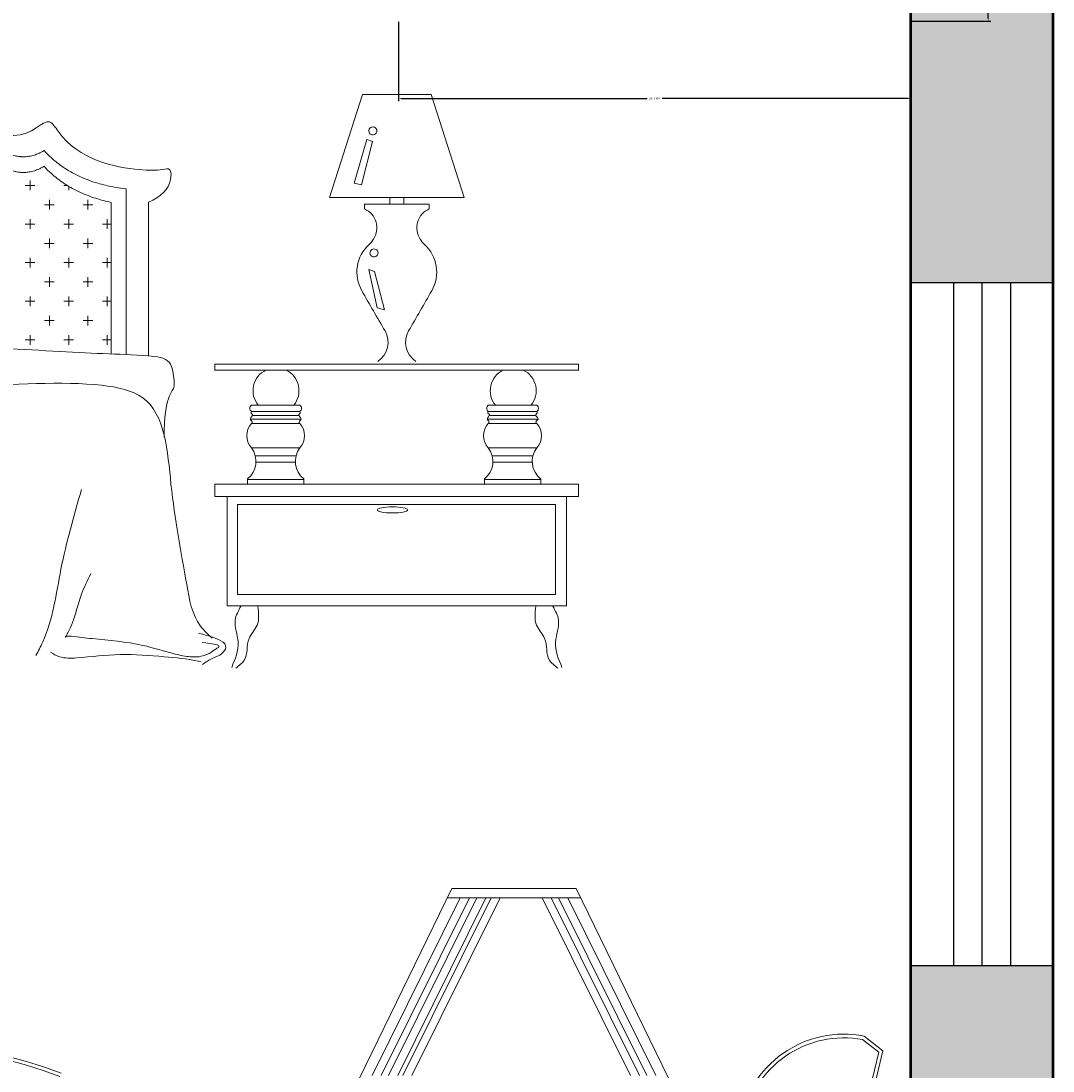
# Model space of a CAD drawing. Units: inches. Extents: x 1771 to 3025, y 319 to 889.
# Tile 34 of 35: x 2952 to 3025, y 714 to 788. Entities that reach past the tile are written whole.
import ezdxf

# ---------------------------------------------------------------- set-up
doc = ezdxf.new("R2010")
doc.units = ezdxf.units.IN
doc.header["$MEASUREMENT"] = 0
doc.set_wipeout_variables(frame=1)
for name, color, linetype, lineweight in [('A-ANNO-DIMS', 2, 'Continuous', 18), ('A-FURN', 8, 'Continuous', 18), ('A-GLAZ', 40, 'Continuous', 25), ('A-WALL', 7, 'Continuous', 50), ('A-WALL-PATT', 254, 'Continuous', 13)]:
    doc.layers.add(name, color=color, linetype=linetype, lineweight=lineweight)
doc.styles.get("Standard").update_dxf_attribs({"font": 'arial.ttf'})
doc.dimstyles.get("Standard").update_dxf_attribs({"dimtxt": 0.18, "dimasz": 0.18, "dimexe": 0.18, "dimexo": 0.0625, "dimgap": 0.09, "dimtad": 0, "dimtih": 1, "dimtoh": 1, "dimdec": 4, "dimzin": 0, "dimdsep": 46, "dimtxsty": 'Standard', "dimcen": 0.09, "dimadec": 0, "dimazin": 0, "dimtfac": 1, "dimtdec": 4, "dimtofl": 0, "dimtmove": 0, "dimatfit": 3, "dimfxl": 1, "dimtolj": 1, "dimtzin": 0, "dimarcsym": 0})

# ---------------------------------------------------------------- blocks, each defined once
blk = doc.blocks.new('A$C3F6F0378')
for p, q in [((2294.6, 774.2), (2348.7, 943.6)), ((2462.2, 943.6), (2348.7, 943.6)), ((2516.4, 774.2), (2462.2, 943.6)), ((2335.1, 797.8), (2356.3, 869.3)), ((2365.5, 866.2), (2347.3, 794.8)), ((2356.3, 869.3), (2365.5, 866.2)), ((1801.9, 785.9), (1801.9, 801.8)), ((2347.3, 794.8), (2335.1, 797.8)), ((1794, 793.9), (1809.9, 793.9)), ((1857.5, 793.9), (1863, 793.9)), ((1865.4, 785.9), (1865.4, 792.4)), ((1825.7, 762.1), (1841.6, 762.1)), ((1833.7, 754.2), (1833.7, 770)), ((1889.2, 762.1), (1905.1, 762.1)), ((1897.2, 754.2), (1897.2, 770)), ((2516.4, 774.2), (2294.6, 774.2)), ((2352.3, 763), (2352.3, 755.2)), ((2352.3, 763), (2352.3, 755.2)), ((2458.6, 763), (2352.3, 763)), ((2393.8, 774.2), (2393.8, 763)), ((2417.1, 763), (2393.8, 763)), ((2417.1, 774.2), (2417.1, 763)), ((2458.6, 763), (2458.6, 755.2)), ((2458.6, 763), (2458.6, 755.2)), ((1794, 730.4), (1809.9, 730.4)), ((1801.9, 722.4), (1801.9, 738.3)), ((1857.5, 730.4), (1873.4, 730.4)), ((1865.4, 722.4), (1865.4, 738.3)), ((1921, 730.4), (1935.3, 730.4)), ((1928.9, 722.4), (1928.9, 738.3)), ((1825.7, 698.6), (1841.6, 698.6)), ((1833.7, 690.7), (1833.7, 706.5)), ((1889.2, 698.6), (1905.1, 698.6)), ((1897.2, 690.7), (1897.2, 706.5)), ((1801.9, 658.9), (1801.9, 674.8)), ((1865.4, 658.9), (1865.4, 674.8)), ((1928.9, 658.9), (1928.9, 674.8)), ((1794, 666.9), (1809.9, 666.9)), ((1857.5, 666.9), (1873.4, 666.9)), ((1921, 666.9), (1935.3, 666.9)), ((1833.7, 627.2), (1833.7, 643)), ((1897.2, 627.2), (1897.2, 643)), ((2359.5, 655.6), (2368.6, 652.5)), ((2373.2, 592.3), (2359.5, 655.6)), ((2368.6, 652.5), (2385.4, 589.2)), ((1825.7, 635.1), (1841.6, 635.1)), ((1889.2, 635.1), (1905.1, 635.1)), ((1801.9, 595.4), (1801.9, 611.3)), ((1865.4, 595.4), (1865.4, 611.3)), ((1928.9, 595.4), (1928.9, 611.3)), ((1794, 603.4), (1809.9, 603.4)), ((1857.5, 603.4), (1873.4, 603.4)), ((1921, 603.4), (1935.3, 603.4)), ((2385.4, 589.2), (2373.2, 592.3)), ((1825.7, 571.6), (1841.6, 571.6)), ((1833.7, 563.7), (1833.7, 579.5)), ((1889.2, 571.6), (1905.1, 571.6)), ((1897.2, 563.7), (1897.2, 579.5)), ((1794, 539.9), (1809.9, 539.9)), ((1801.9, 531.9), (1801.9, 547.8)), ((1857.5, 539.9), (1873.4, 539.9)), ((1865.4, 531.9), (1865.4, 547.8)), ((1921, 539.9), (1935.3, 539.9)), ((1928.9, 531.9), (1928.9, 547.8)), ((2704.5, 500), (2106.1, 500)), ((2106.1, 499.7), (2106.1, 489.7)), ((2704.5, 490), (2106.1, 490)), ((2704.5, 499.7), (2704.5, 489.7)), ((2246.1, 432.2), (2166.1, 432.2)), ((2246.1, 432.2), (2166.1, 432.2)), ((2635.9, 432.2), (2555.9, 432.2)), ((2635.9, 432.2), (2555.9, 432.2)), ((2246.1, 422.2), (2166.1, 422.2)), ((2244.2, 415.4), (2167.9, 415.4)), ((2635.9, 422.2), (2555.9, 422.2)), ((2634.1, 415.4), (2557.7, 415.4)), ((2248, 409.3), (2164.1, 409.3)), ((2246.1, 402.2), (2166.1, 402.2)), ((2637.9, 409.3), (2554, 409.3)), ((2635.9, 402.2), (2555.9, 402.2)), ((2246.1, 362.2), (2166.1, 362.2)), ((2239.7, 349.2), (2172.4, 349.2)), ((2635.9, 362.2), (2555.9, 362.2)), ((2629.6, 349.2), (2562.2, 349.2)), ((2238.5, 338.7), (2173.6, 338.7)), ((2628.4, 338.7), (2563.5, 338.7)), ((2159.8, 311), (2159.8, 302.2)), ((2252.3, 311), (2252.3, 302.2)), ((2549.7, 311), (2549.7, 302.2)), ((2642.2, 311), (2642.2, 302.2)), ((2106.1, 302.2), (2106.1, 282.2)), ((2704.5, 302.2), (2106.1, 302.2)), ((2252.3, 310.3), (2159.8, 310.3)), ((2186.1, 302.2), (2226.1, 302.2)), ((2186.1, 302.2), (2236.1, 302.2)), ((2642.2, 310.3), (2549.7, 310.3)), ((2575.9, 302.2), (2615.9, 302.2)), ((2575.9, 302.2), (2625.9, 302.2)), ((2704.5, 282.2), (2704.5, 302.2)), ((2704.5, 282.2), (2106.1, 282.2)), ((2126.1, 282.2), (2126.1, 102.2)), ((2684.5, 102.2), (2684.5, 282.2)), ((2143.3, 268.9), (2666.3, 268.9)), ((2143.3, 120.8), (2143.3, 268.9)), ((2666.3, 268.9), (2666.3, 120.8)), ((2666.3, 120.8), (2143.3, 120.8)), ((2126.1, 102.2), (2684.5, 102.2))]:
    blk.add_line(p, q)
at = {"ltscale": 20}
for p, q in [((1959.8, 788.3), (1959.8, 515.7)), ((1935.3, 766), (1935.3, 516.7)), ((1996.6, 766.2), (1996.6, 513.5))]:
    blk.add_line(p, q, dxfattribs=at)
for centre, radius, start, end in [((2365.7, 883.6), 6.48, 168.6084, 233.2112), ((2365.7, 883.6), 6.49, 104.0344, 168.6084), ((2366.1, 883.6), 6.51, 78.6968, 107.1924), ((2365.7, 883.9), 6.81, 278.2688, 342.9026), ((2366.1, 883.7), 6.5, 50.1648, 78.6968), ((2366.2, 883.8), 6.35, 342.9026, 50.1648), ((2365.7, 883.5), 6.42, 233.2112, 255.9722), ((2365.7, 883.8), 6.69, 255.9722, 278.2688), ((2338.7, 724.1), 33.9, 326.6744, 66.3416), ((2472.2, 724.1), 33.9, 113.6584, 213.3256), ((2401.2, 651.2), 61.5, 132.0366, 209.8723), ((2337, 722.3), 34.4, 312.0366, 330.6067), ((2473.8, 722.3), 34.4, 209.3933, 227.9634), ((2409.6, 651.2), 61.5, 330.1277, 47.9634), ((2367.7, 682.8), 6.48, 168.6084, 233.2112), ((2367.7, 682.8), 6.49, 104.0344, 168.6084), ((2367.7, 682.8), 6.42, 233.2112, 255.9722), ((2367.8, 683), 6.69, 255.9722, 278.2688), ((2368.1, 682.9), 6.51, 78.6968, 107.1924), ((2367.8, 683.1), 6.81, 278.2688, 342.9026), ((2368.1, 682.9), 6.5, 50.1648, 78.6968), ((2368.2, 683), 6.35, 342.9026, 50.1648), ((11218.8, 5715.8), 10230.1, 209.87228, 210.29853), ((-6408, 5715.8), 10230.1, 329.70147, 330.12772), ((2353.9, 535.9), 37.3, 302.5427, 30.2985), ((2457, 535.9), 37.3, 149.7015, 237.4573), ((2206.6, 456.1), 37.8, 115.9414, 219.2084), ((2206.6, 456.1), 37.8, 320.7916, 64.0586), ((2597, 456.1), 37.8, 115.9414, 219.2084), ((2597, 456.1), 37.8, 320.7916, 64.0586), ((2169.8, 427.2), 6.24, 126.78, 233.22), ((2242.3, 427.2), 6.24, 306.78, 53.22), ((2559.7, 427.2), 6.24, 126.78, 233.22), ((2632.2, 427.2), 6.24, 306.78, 53.22), ((2188.1, 382.2), 29.7, 137.7452, 222.2548), ((2224, 382.2), 29.7, 317.7452, 42.2548), ((2577.9, 382.2), 29.7, 137.7452, 222.2548), ((2613.9, 382.2), 29.7, 317.7452, 42.2548), ((2136.7, 339.8), 37, 308.7547, 37.2668), ((2275.4, 339.8), 37, 142.7332, 231.2453), ((2526.5, 339.8), 37, 308.7547, 37.2668), ((2665.3, 339.8), 37, 142.7332, 231.2453)]:
    blk.add_arc(centre, radius, start, end)
blk.add_ellipse((2398.3, 260.1), major_axis=(25, 0), ratio=0.2)
for points, knots in [([(1996.6, 766.2), (2017.1, 775.8), (2035.1, 791.6), (2033.8, 824.3), (2016.6, 817.9), (1960.4, 819.9), (1874.7, 836.7), (1829, 913.8), (1803, 869.9), (1652.5, 896.6), (1584, 1003.6), (1395.1, 1025), (1329.4, 1035.8)], [12.417853, 12.417853, 12.417853, 12.417853, 68.394536, 90.665986, 114.156853, 157.554067, 281.869614, 298.858744, 338.737111, 347.060176, 470.423438, 625.498764, 625.498764, 625.498764, 625.498764]), ([(1824.9, 851.3), (1824.2, 850.9), (1823.5, 850.4), (1821.1, 849.1), (1819.5, 848.2), (1815.6, 846.3), (1813.3, 845.4), (1808.4, 843.6), (1805.7, 842.8), (1800.3, 841.7), (1797.7, 841.4), (1794, 841.1), (1792.9, 841), (1791.2, 841), (1790.5, 841), (1789.2, 841), (1788.6, 841.1), (1787.5, 841.1), (1787, 841.2), (1785.3, 841.3), (1784.3, 841.4), (1780.8, 841.9), (1778.6, 842.3), (1774.6, 843.3), (1772.8, 843.9), (1769.6, 844.9), (1768.2, 845.5), (1765.8, 846.4), (1764.7, 846.9), (1763.5, 847.4), (1763.2, 847.5), (1762.7, 847.8), (1762.4, 847.9), (1761.6, 848.2), (1761.1, 848.5), (1759.5, 849.2), (1758.4, 849.7), (1755.2, 851.3), (1753.2, 852.3), (1664.6, 855.5), (1660.7, 857.8), (1650.1, 864.4), (1643.7, 869), (1631.7, 878.3), (1626.1, 883.1), (1615.5, 892.7), (1610.4, 897.5), (1600.8, 907), (1596.2, 911.6), (1587.3, 920.6), (1583, 924.9), (1574.7, 933), (1570.6, 936.8), (1492.6, 942), (1490.8, 943.5), (1487.5, 946.3), (1486.1, 947.4), (1483.8, 949.2), (1482.9, 949.9), (1481.1, 951.2), (1480.2, 951.8), (1477.4, 953.8), (1475.5, 955), (1469.8, 958.7), (1465.9, 961), (1454.8, 967), (1447.3, 970.4), (1431.5, 976.7), (1423.2, 979.5), (1405.8, 984.7), (1396.8, 987), (1378.1, 991.3), (1368.4, 993.3), (1349, 996.9), (1339.3, 998.6), (1329.5, 1000.2)], [328.6705, 328.6705, 328.6705, 328.6705, 329.609368, 329.609368, 331.487103, 331.487103, 333.620342, 333.620342, 335.753581, 335.753581, 337.507866, 337.507866, 338.182373, 338.182373, 338.607397, 338.607397, 338.959312, 338.959312, 339.311227, 339.311227, 340.015058, 340.015058, 341.722742, 341.722742, 343.430427, 343.430427, 345.138111, 345.138111, 346.845796, 346.845796, 347.37881, 347.37881, 347.911824, 347.911824, 348.977853, 348.977853, 351.109909, 351.109909, 355.374023, 355.374023, 363.902249, 363.902249, 379.258481, 379.258481, 394.614712, 394.614712, 409.970943, 409.970943, 425.327175, 425.327175, 440.683406, 440.683406, 456.039637, 456.039637, 463.285514, 463.285514, 469.011154, 469.011154, 472.592992, 472.592992, 476.17483, 476.17483, 483.338506, 483.338506, 497.665857, 497.665857, 522.309275, 522.309275, 546.952693, 546.952693, 571.59611, 571.59611, 596.239528, 596.239528, 619.876409, 619.876409, 619.876409, 619.876409]), ([(1824.9, 825.4), (1824.2, 825), (1823.5, 824.6), (1821.1, 823.2), (1819.5, 822.3), (1815.6, 820.5), (1813.3, 819.5), (1808.4, 817.8), (1805.7, 817), (1800.3, 815.9), (1797.7, 815.5), (1794, 815.2), (1792.9, 815.2), (1791.2, 815.2), (1790.5, 815.2), (1789.2, 815.2), (1788.6, 815.2), (1787.5, 815.3), (1787, 815.3), (1785.3, 815.4), (1784.3, 815.5), (1780.8, 816), (1778.6, 816.5), (1774.6, 817.5), (1772.8, 818), (1769.6, 819.1), (1768.2, 819.6), (1765.8, 820.6), (1764.7, 821), (1763.5, 821.5), (1763.2, 821.7), (1762.7, 821.9), (1762.4, 822), (1761.6, 822.4), (1761.1, 822.6), (1759.5, 823.4), (1758.4, 823.9), (1755.2, 825.4), (1753.2, 826.4), (1664.6, 829.7), (1660.7, 832), (1650.1, 838.6), (1643.7, 843.1), (1631.7, 852.4), (1626.1, 857.2), (1615.5, 866.8), (1610.4, 871.6), (1600.8, 881.1), (1596.2, 885.7), (1587.3, 894.7), (1583, 899), (1574.7, 907.1), (1570.6, 910.9), (1492.6, 916.1), (1490.8, 917.7), (1487.5, 920.4), (1486.1, 921.5), (1483.8, 923.3), (1482.9, 924), (1481.1, 925.3), (1480.2, 926), (1477.4, 927.9), (1475.5, 929.2), (1469.8, 932.8), (1465.9, 935.2), (1454.8, 941.1), (1447.3, 944.6), (1431.5, 950.8), (1423.2, 953.7), (1405.8, 958.8), (1396.8, 961.2), (1378.1, 965.5), (1368.4, 967.4), (1349, 971), (1339.3, 972.7), (1329.5, 974.3)], [328.6705, 328.6705, 328.6705, 328.6705, 329.609368, 329.609368, 331.487103, 331.487103, 333.620342, 333.620342, 335.753581, 335.753581, 337.507866, 337.507866, 338.182373, 338.182373, 338.607397, 338.607397, 338.959312, 338.959312, 339.311227, 339.311227, 340.015058, 340.015058, 341.722742, 341.722742, 343.430427, 343.430427, 345.138111, 345.138111, 346.845796, 346.845796, 347.37881, 347.37881, 347.911824, 347.911824, 348.977853, 348.977853, 351.109909, 351.109909, 355.374023, 355.374023, 363.902249, 363.902249, 379.258481, 379.258481, 394.614712, 394.614712, 409.970943, 409.970943, 425.327175, 425.327175, 440.683406, 440.683406, 456.039637, 456.039637, 463.285514, 463.285514, 469.011154, 469.011154, 472.592992, 472.592992, 476.17483, 476.17483, 483.338506, 483.338506, 497.665857, 497.665857, 522.309275, 522.309275, 546.952693, 546.952693, 571.59611, 571.59611, 596.239528, 596.239528, 619.876409, 619.876409, 619.876409, 619.876409]), ([(1959.8, 788.3), (1947.6, 789.5), (1939.9, 790.9), (1923.7, 794.5), (1915.4, 796.7), (1898.5, 802.3), (1889.9, 805.7), (1873, 813.7), (1864.6, 818.4), (1849.7, 828.5), (1843.2, 833.6), (1832.8, 843.1), (1828.8, 847.1), (1824.9, 851.3)], [179.400376, 179.400376, 179.400376, 179.400376, 196.086144, 196.086144, 213.445516, 213.445516, 230.804888, 230.804888, 248.16426, 248.16426, 262.451931, 262.451931, 271.832526, 271.832526, 271.832526, 271.832526]), ([(1935.3, 766), (1934.2, 766.3), (1933.1, 766.5), (1923.7, 768.6), (1915.4, 770.9), (1898.5, 776.5), (1889.9, 779.8), (1873, 787.9), (1864.6, 792.6), (1849.7, 802.7), (1843.2, 807.8), (1832.8, 817.2), (1828.8, 821.2), (1824.9, 825.4)], [193.740688, 193.740688, 193.740688, 193.740688, 196.086144, 196.086144, 213.445516, 213.445516, 230.804888, 230.804888, 248.16426, 248.16426, 262.451931, 262.451931, 271.832526, 271.832526, 271.832526, 271.832526])]:
    blk.add_open_spline(points, degree=3, knots=knots, dxfattribs=at)
at = {"ltscale": 5}
for points, knots in [([(2022.3, 380), (2023.2, 448.3), (2041.3, 454.3), (2037.8, 480.9), (2034.7, 509.9), (1981.7, 515.4), (1909.3, 516.7), (1667.8, 533.2), (1476.1, 527.9), (1347.4, 530.2)], [0, 0, 0, 0, 32.681627, 48.455722, 75.25348, 112.004017, 183.381957, 310.642358, 588.939547, 588.939547, 588.939547, 588.939547]), ([(2101.8, 49), (2094.8, 55.3), (2069.8, 78.1), (2053.9, 172), (2031.7, 287.1), (2023.3, 445.1), (1887.5, 475), (1637.7, 455.3), (1416.4, 458.5), (1314.5, 461.4)], [0, 0, 0, 0, 28.320233, 100.953775, 269.820348, 420.691469, 489.161544, 656.134073, 940.569207, 940.569207, 940.569207, 940.569207]), ([(1886.4, 293.6), (1874, 250.4), (1850.2, 167.7), (1838.6, 71.7), (1815.4, 27.8), (1811.5, 20.4)], [0, 0, 0, 0, 135.247847, 258.692787, 283.800228, 283.800228, 283.800228, 283.800228]), ([(1901.7, 155.1), (1896.3, 144.1), (1881.1, 112.8), (1874.4, 74.6), (1861.4, 53), (1859.9, 50.7)], [0, 0, 0, 0, 37.234018, 105.386078, 113.844905, 113.844905, 113.844905, 113.844905]), ([(2080.3, 18.4), (2075.6, 18.3), (2062.2, 17.9), (2030.9, 24.9), (1978.8, 41.9), (1919.5, 46.5), (1879.3, 50.9), (1863, 53.1), (1860.4, 51), (1859.9, 50.7)], [0, 0, 0, 0, 14.447875, 40.468341, 96.220884, 181.018327, 216.046098, 224.609189, 226.185962, 226.185962, 226.185962, 226.185962]), ([(2079, 57.4), (2084.9, 55.8), (2100.2, 51.8), (2131, 40.6), (2116.7, 21.1), (2101.3, 16.6), (2091, 9.7), (2085.5, 5.9)], [0, 0, 0, 0, 19.937155, 51.57724, 63.193909, 80.21631, 100.09061, 100.09061, 100.09061, 100.09061]), ([(2084.9, 41.8), (2100.9, 40.1), (2120.5, 38.1), (2104.4, 29.7), (2095.5, 21.9), (2085.1, 19.8), (2078.6, 18.4)], [0, 0, 0, 0, 28.05485, 34.289435, 45.980108, 65.027556, 65.027556, 65.027556, 65.027556]), ([(2083.5, 9.9), (2082, 10.3), (2061.3, 15.5), (2017.8, 18.7), (1949.9, 25.1), (1893.7, 17), (1853.5, 15.4), (1840.4, 23.1), (1835.5, 26)], [590.079786, 590.079786, 590.079786, 590.079786, 594.646549, 651.888327, 725.747367, 797.841373, 826.274406, 843.189267, 843.189267, 843.189267, 843.189267])]:
    blk.add_open_spline(points, degree=3, knots=knots, dxfattribs=at)
for points, knots in [([(2166.1, 422.2), (2165.6, 421), (2164.6, 418.8), (2169.4, 417.1), (2166.2, 412.9), (2162.3, 408.7), (2169.1, 405.7), (2166.9, 403.1), (2166.1, 402.2)], [0, 0, 0, 0, 3.125, 6.207289, 10.622222, 14.901958, 20.470919, 23.596268, 23.596268, 23.596268, 23.596268]), ([(2246, 422.2), (2246.5, 421), (2247.5, 418.8), (2242.7, 417.1), (2245.9, 412.9), (2249.8, 408.7), (2243, 405.7), (2245.2, 403.1), (2246, 402.2)], [0, 0, 0, 0, 3.125, 6.207289, 10.622222, 14.901958, 20.470919, 23.596268, 23.596268, 23.596268, 23.596268]), ([(2555.9, 422.2), (2555.5, 421), (2554.5, 418.8), (2559.3, 417.1), (2556.1, 412.9), (2552.2, 408.7), (2559, 405.7), (2556.7, 403.1), (2555.9, 402.2)], [0, 0, 0, 0, 3.125, 6.207289, 10.622222, 14.901958, 20.470919, 23.596268, 23.596268, 23.596268, 23.596268]), ([(2635.9, 422.2), (2636.4, 421), (2637.3, 418.8), (2632.5, 417.1), (2635.8, 412.9), (2639.7, 408.7), (2632.8, 405.7), (2635.1, 403.1), (2635.9, 402.2)], [0, 0, 0, 0, 3.125, 6.207289, 10.622222, 14.901958, 20.470919, 23.596268, 23.596268, 23.596268, 23.596268]), ([(2148.9, 101.6), (2144.7, 94.2), (2134.2, 75.7), (2149.9, 40.1), (2139.4, 14.7), (2133.7, 0.9)], [0, 0, 0, 0, 24.696996, 61.099524, 104.177437, 104.177437, 104.177437, 104.177437]), ([(2176.5, 101.6), (2178, 90.6), (2180.7, 70.5), (2155.8, 47.4), (2161.8, 15.4), (2145.9, 4), (2140.4, 0)], [0, 0, 0, 0, 31.35672, 56.935761, 92.890491, 112.386558, 112.386558, 112.386558, 112.386558]), ([(2634.4, 101.6), (2632.9, 90.6), (2630.2, 70.5), (2655.1, 47.4), (2649.1, 15.4), (2665, 4), (2670.5, 0)], [0, 0, 0, 0, 31.35672, 56.935761, 92.890491, 112.386558, 112.386558, 112.386558, 112.386558]), ([(2662, 101.6), (2666.2, 94.2), (2676.7, 75.7), (2661, 40.1), (2671.5, 14.7), (2677.2, 0.9)], [0, 0, 0, 0, 24.696996, 61.099524, 104.177437, 104.177437, 104.177437, 104.177437])]:
    blk.add_open_spline(points, degree=3, knots=knots)
blk = doc.blocks.new('A$C425441F1')
for points in [[(1639.3, 0), (1667.3, 0), (1667.3, 55.3), (1748.6, 55.3), (1748.6, 807.4), (1761.1, 860.7), (1735.7, 880.7), (1703.4, 883.3), (1675.8, 879.6), (1656.2, 873.5), (1635.2, 863.3), (1619.6, 852.6), (1605.1, 839.5), (1596.7, 829.9), (1583.2, 810), (1573.2, 788.1), (1567.6, 767.7), (1566.5, 761.6), (1541.6, 750.9), (1510.7, 736.6), (1488.3, 725.3), (1464.5, 712.2), (1433.4, 693.6), (1409.1, 677.8), (1389.7, 664.2), (1388.2, 683.8), (1383.3, 700), (1376.2, 712), (1365.5, 723.2), (1352, 731.8), (1342.1, 735.4), (1331.7, 738.6), (1325, 742.7), (1317.7, 750.9), (1314.2, 758.8), (1312.9, 767.9), (1315.6, 780.8), (1321.1, 788.9), (1323.4, 793.7), (1323.6, 797.2), (1323.1, 800), (1320.5, 804.5), (1317.8, 806.7), (1317.8, 807.1), (1478.8, 807.1), (1345.8, 1080.7), (1177.3, 1080.7), (1044.3, 807.1), (1211.1, 807.1), (1211.1, 806.7), (1207.8, 803.9), (1205.8, 800.4), (1205.1, 796.3), (1207.6, 788.9), (1211.4, 783.4), (1213.5, 778.7), (1215.3, 769.8), (1215.1, 763.9), (1214.1, 759), (1208.8, 748.5), (1201.9, 741.7), (1195.3, 738), (1185.9, 735.4), (1176, 731.7), (1166.8, 726.4), (1159.9, 720.8), (1156.8, 717.7), (1149.3, 708.1), (1145.7, 701.6), (1143.6, 696.9), (1138.7, 669.7), (1138.7, 651.6), (1140.7, 631.8), (1142.6, 621.6), (1148.5, 600.5), (1162.8, 569), (1176.9, 547.8), (1188.6, 534.2), (1200, 523), (983, 523), (977.7, 522.3), (971.8, 519.6), (965.5, 512.8), (963.3, 506.8), (963, 503), (974.8, 503), (974.8, 3), (1013, 3), (1013, 103), (1053.6, 103), (1052.7, 96.1), (1051.6, 86.5), (1049.3, 63.6), (1048.6, 55.3), (1130.1, 55.3), (1130.1, 0), (1157.9, 0), (1174.1, 55.3), (1623.1, 55.6)], [(778.6, 0), (750.6, 0), (750.6, 50.4), (141.4, 50.4), (141.4, 0), (113.4, 0), (98.1, 50.4), (0, 50.4), (0, 590.4), (3.6, 609.1), (14.7, 633.7), (36.6, 658.7), (60.6, 673.3), (86.6, 680.5), (100.5, 681.5), (107.8, 698), (118.3, 717), (136.4, 751.3), (159.1, 779.5), (188.4, 803.6), (213.2, 817.4), (239.4, 827.1), (258.7, 831.4), (276, 833.4), (301.1, 842.1), (332.2, 850.9), (368.4, 858.6), (403.3, 863.5), (432.7, 865.8), (472.6, 866.2), (499.3, 864.8), (525, 862.1), (551.9, 857.9), (572.9, 853.6), (591.1, 849.1), (612.6, 842.8), (648, 830.4), (661.5, 823.7), (679.5, 815.2), (707.5, 798.2), (726.7, 783.3), (755.4, 754.4), (773.7, 729.8), (788.1, 704.9), (796.6, 686.1), (798.5, 681.2), (818, 677.9), (833.5, 672.3), (851.7, 661.6), (864.4, 650.3), (878.3, 632.1), (887.5, 611.7), (891.4, 595.2), (892, 590.4), (892, 50.4), (793.9, 50.4)]]:
    blk.add_wipeout(points)
for p, q in [((1044.3, 807.1), (1177.3, 1080.7)), ((1177.3, 1080.7), (1044.3, 807.1)), ((1177.3, 1080.7), (1345.8, 1080.7)), ((1345.8, 1080.7), (1177.3, 1080.7)), ((1345.8, 1080.7), (1478.8, 807.1)), ((1478.8, 807.1), (1345.8, 1080.7)), ((1188.8, 1068), (1069.3, 827.4)), ((1201.1, 1068), (1081.6, 827.4)), ((1211.2, 1068), (1091.7, 827.4)), ((1223.5, 1068), (1104, 827.4)), ((1230.5, 1068), (1110.9, 827.4)), ((1242.8, 1068), (1123.2, 827.4)), ((1171, 1067.8), (1351.9, 1067.8)), ((1299.6, 1068), (1419.2, 827.4)), ((1311.9, 1068), (1431.5, 827.4)), ((1322, 1068), (1441.5, 827.4)), ((1334.3, 1068), (1453.8, 827.4)), ((1733.6, 876.1), (1755.5, 858.7)), ((1735.7, 880.7), (1761.1, 860.7)), ((1744.1, 810.1), (1755.5, 858.7)), ((1748.6, 807.4), (1761.1, 860.7))]:
    blk.add_line(p, q)
for centre, radius, start, end in [((1708.4, 739.8), 143.6, 79.0486, 171.2543), ((1708.4, 739.8), 138.6, 79.5487, 170.0411), ((458.1, 348.7), 517.8, 68.4843, 110.5916), ((458.1, 348.7), 512.8, 68.4843, 110.5916)]:
    blk.add_arc(centre, radius, start, end)
blk = doc.blocks.new('WIN-48')
for p, q in [((0, 0), (0, 10)), ((48, 0), (48, 10)), ((0, 7), (48, 7)), ((0, 5), (48, 5)), ((0, 3), (48, 3))]:
    blk.add_line(p, q)
blk = doc.blocks.new('*D30')
at = {"layer": 'A-ANNO-DIMS', "color": 0, "lineweight": -2, "transparency": 16777216}
for p, q in [((3014.747, 824.128), (3020.309, 824.128)), ((3020.129, 823.948), (3020.129, 806.162)), ((3020.129, 788.01), (3020.129, 805.796)), ((3014.747, 787.83), (3020.309, 787.83))]:
    blk.add_line(p, q, dxfattribs=at)
at = {"layer": 'A-ANNO-DIMS', "color": 0, "transparency": 16777216}
for points in [[(3020.099, 823.948), (3020.159, 823.948), (3020.129, 824.128)], [(3020.099, 788.01), (3020.159, 788.01), (3020.129, 787.83)]]:
    blk.add_solid(points, dxfattribs=at)
at = {"layer": 'Defpoints', "color": 0, "transparency": 16777216}
for p in [(3014.685, 824.128), (3020.129, 824.128), (3014.685, 787.83)]:
    blk.add_point(p, dxfattribs=at)
at = {"layer": 'A-ANNO-DIMS', "color": 0, "transparency": 16777216, "insert": (3020.129, 805.979), "char_height": 0.18, "attachment_point": 5}
blk.add_mtext('\\A1;DOOR D2 36 TYP.', dxfattribs=at)
blk = doc.blocks.new('*D31')
at = {"layer": 'A-ANNO-DIMS', "color": 0, "lineweight": -2, "transparency": 16777216}
for p, q in [((2978.685, 787.768), (2978.685, 782.206)), ((3014.685, 787.768), (3014.685, 782.206)), ((2978.865, 782.386), (2996.157, 782.386)), ((3014.505, 782.386), (2997.213, 782.386))]:
    blk.add_line(p, q, dxfattribs=at)
at = {"layer": 'A-ANNO-DIMS', "color": 0, "transparency": 16777216}
for points in [[(2978.865, 782.416), (2978.865, 782.356), (2978.685, 782.386)], [(3014.505, 782.416), (3014.505, 782.356), (3014.685, 782.386)]]:
    blk.add_solid(points, dxfattribs=at)
at = {"layer": 'Defpoints', "color": 0, "transparency": 16777216}
for p in [(2978.685, 787.83), (3014.685, 787.83), (3014.685, 782.386)]:
    blk.add_point(p, dxfattribs=at)
at = {"layer": 'A-ANNO-DIMS', "color": 0, "transparency": 16777216, "insert": (2996.685, 782.386), "char_height": 0.18, "attachment_point": 5}
blk.add_mtext('\\A1;36 TYP.', dxfattribs=at)

msp = doc.modelspace()

# ---------------------------------------------------------------- hatches: boundary and pattern name
at = {"layer": 'A-WALL-PATT'}
h = msp.add_hatch(color=256, dxfattribs=at)
h.dxf.hatch_style = 1
h.paths.add_polyline_path([(2870.685, 879.484), (2892.728, 879.484), (2892.728, 889.484), (2842.685, 889.484), (2842.685, 879.484), (2865.685, 879.484), (2865.685, 831.484), (2870.685, 831.484)])
h.paths.add_polyline_path([(2983.637, 889.484), (2940.728, 889.484), (2940.728, 879.484), (2961.685, 879.484), (2961.685, 795.484), (2865.685, 795.484), (2865.685, 759.484), (2865.685, 665.484), (2870.685, 665.484), (2870.685, 712.85), (2870.685, 790.484), (2978.685, 790.484), (2978.685, 795.484), (2966.685, 795.484), (2966.685, 879.484), (2983.637, 879.484)])
h.paths.add_polyline_path([(3024.685, 889.484), (3001.637, 889.484), (3001.637, 879.484), (3014.685, 879.484), (3014.685, 790.484), (3014.685, 769.459), (3024.685, 769.459)])
h.paths.add_polyline_path([(3024.685, 721.459), (3014.685, 721.459), (3014.685, 670.484), (2906.685, 670.484), (2906.685, 665.484), (2925.685, 665.484), (2925.685, 653.484), (2930.685, 653.484), (2930.685, 665.484), (3014.685, 665.484), (3014.685, 650.024), (3024.685, 650.024)])
h.paths.add_polyline_path([(3024.685, 632.024), (3014.685, 632.024), (3014.685, 617.484), (2925.685, 617.484), (2906.685, 617.484), (2906.685, 612.484), (3014.685, 612.484), (3014.685, 581.957), (3024.685, 581.957)])
h.paths.add_polyline_path([(3024.685, 533.957), (3014.685, 533.957), (3014.685, 480.484), (2870.685, 480.484), (2870.685, 617.484), (2860.685, 617.484), (2860.685, 544.484), (2769.685, 544.484), (2769.685, 534.484), (2860.685, 534.484), (2860.685, 470.484), (3014.685, 470.484), (3014.685, 453.613), (3024.685, 453.613)])
h.paths.add_polyline_path([(3024.685, 405.613), (3014.685, 405.613), (3014.685, 394.484), (2860.685, 394.484), (2860.685, 384.484), (3024.685, 384.484)])
h.paths.add_polyline_path([(2733.685, 643.435), (2723.685, 643.435), (2723.685, 534.484), (2733.685, 534.484)])
h.paths.add_polyline_path([(2733.685, 754.484), (2829.685, 754.484), (2829.685, 759.484), (2733.685, 759.484), (2733.685, 843.439, -0.008336), (2732.382, 843.484), (2723.685, 843.484), (2723.685, 691.435), (2733.685, 691.435)])
h.paths.add_polyline_path([(2794.685, 889.484), (2723.685, 889.484), (2723.685, 879.484), (2794.685, 879.484)])

# ---------------------------------------------------------------- linework, layer by layer
at = {"layer": 'A-WALL'}
for p, q in [((3024.685, 384.484), (3024.685, 889.282)), ((3014.685, 670.484), (3014.685, 790.484))]:
    msp.add_line(p, q, dxfattribs=at)

# ---------------------------------------------------------------- block references
at = {"layer": 'A-FURN', "xscale": 0.0427162254345911, "yscale": 0.0427162254345911, "zscale": 0.0427162254345911}
msp.add_blockref('A$C3F6F0378', (2875.807, 742.363), dxfattribs=at)
at = {"layer": 'A-GLAZ', "rotation": 270.0000000000027}
msp.add_blockref('WIN-48', (3014.685, 769.459), dxfattribs=at)

# ---------------------------------------------------------------- dimensions: what is measured, and where the dimension line sits
at = {"layer": 'A-ANNO-DIMS'}
dim = msp.add_linear_dim(base=(3020.129, 824.128), p1=(3014.685, 787.83), p2=(3014.685, 824.128), angle=90, text='DOOR D2 <> TYP.', dimstyle='Standard', override={"dimdec": 0, "dimrnd": 0, "dimzin": 0, "dimlunit": 2}, dxfattribs=at)
dim.commit()
dim.dimension.update_dxf_attribs({"geometry": '*D30', "text_midpoint": (3020.129, 805.979)})
dim = msp.add_linear_dim(base=(3014.685, 782.386), p1=(2978.685, 787.83), p2=(3014.685, 787.83), text='<> TYP.', dimstyle='Standard', override={"dimdec": 0, "dimrnd": 0, "dimzin": 0, "dimlunit": 2}, dxfattribs=at)
dim.commit()
dim.dimension.update_dxf_attribs({"geometry": '*D31', "text_midpoint": (2996.685, 782.386)})

# ---------------------------------------------------------------- next in the draw order: block references
at = {"layer": 'A-FURN', "xscale": 0.0519011286993662, "yscale": 0.0519011286993662, "zscale": 0.0519011286993662}
msp.add_blockref('A$C425441F1', (2921.321, 670.788), dxfattribs=at)

doc.saveas('drawing.dxf')
